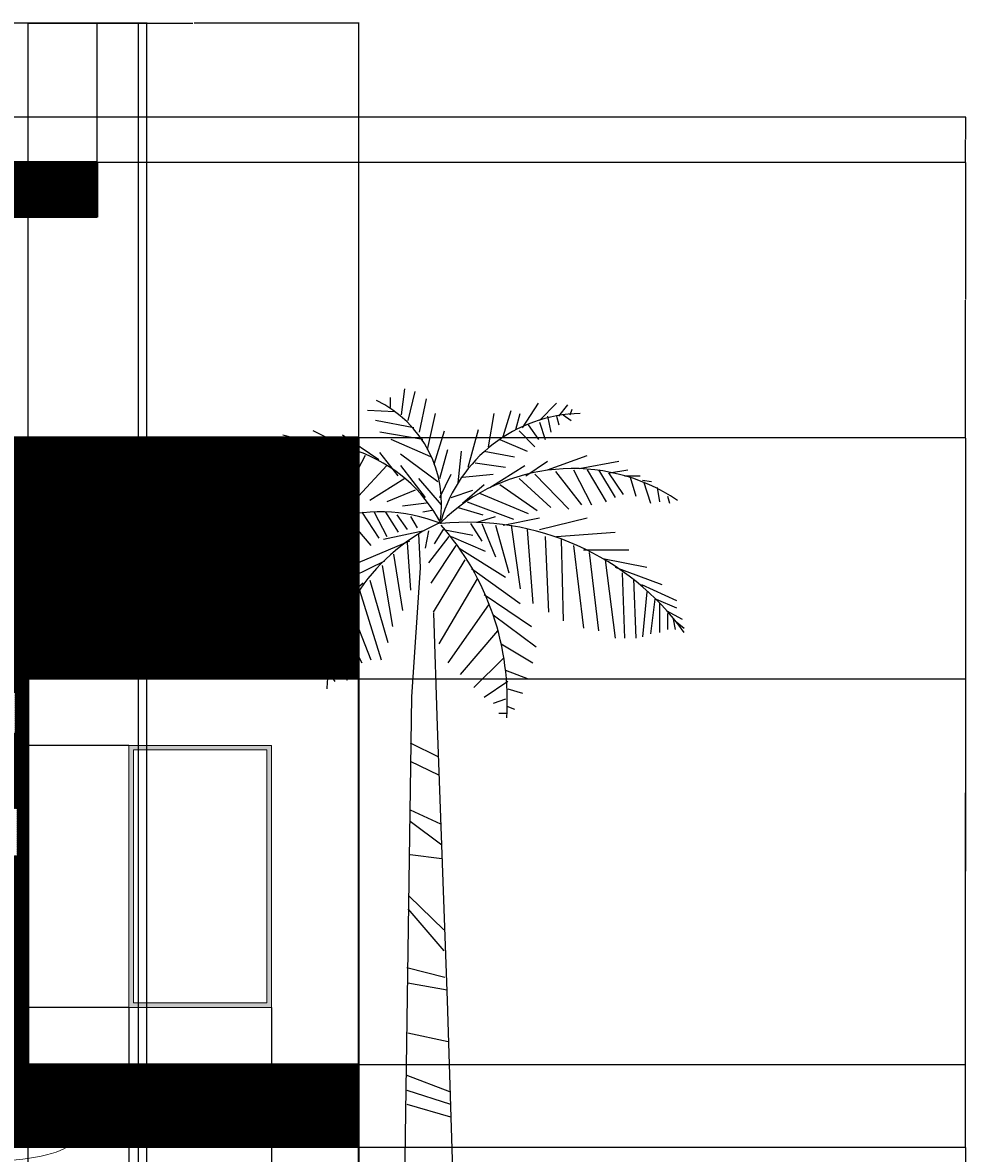
# Model space of a CAD drawing. Units: inches. Extents: x 484 to 1264, y 95 to 991.
# Tile 8 of 8: x 853 to 1264, y 499 to 991. Entities that reach past the tile are written whole.
import ezdxf

# ---------------------------------------------------------------- set-up
doc = ezdxf.new("R2010")
doc.units = ezdxf.units.IN
doc.header["$MEASUREMENT"] = 0
for name, color, linetype, lineweight in [('A-ANNO-DIMS', 2, 'Continuous', 18), ('A-ELEV-TRIM', 7, 'Continuous', 18), ('A-GLAZ', 7, 'Continuous', 18), ('A-WALL', 7, 'Continuous', 35)]:
    doc.layers.add(name, color=color, linetype=linetype, lineweight=lineweight)
doc.layers.add('A-ELEV-TRIM-PATT', color=40, linetype='Continuous', lineweight=13, true_color=0xe7c208)
doc.layers.add('A-WALL-FRAM-PATT', color=158, linetype='Continuous', lineweight=13, true_color=0x131d3e)
doc.layers.add('TREES', color=92, linetype='Continuous')
doc.styles.get("Standard").update_dxf_attribs({"font": 'arial.ttf'})
doc.dimstyles.get("Standard").update_dxf_attribs({"dimtxt": 0.18, "dimasz": 0.18, "dimexe": 0.18, "dimexo": 0.0625, "dimgap": 0.09, "dimtad": 0, "dimtih": 1, "dimtoh": 1, "dimdec": 4, "dimzin": 0, "dimdsep": 46, "dimtxsty": 'Standard', "dimcen": 0.09, "dimadec": 0, "dimazin": 0, "dimtfac": 1, "dimtdec": 4, "dimtofl": 0, "dimtmove": 0, "dimatfit": 3, "dimfxl": 1, "dimtolj": 1, "dimtzin": 0, "dimarcsym": 0})

# ---------------------------------------------------------------- blocks, each defined once
blk = doc.blocks.new('*U3')
for p, q in [((-5.567, 196.707), (-4.987, 201.167)), ((-7.5, 199.68), (-7.5, 197.946)), ((-4.407, 195.716), (-3.247, 200.672)), ((-2.474, 193.733), (-1.315, 199.433)), ((-6.727, 197.202), (-11.366, 197.45)), ((11.829, 192.99), (13.182, 197.45)), ((15.116, 194.477), (17.822, 198.689)), ((18.015, 195.716), (20.914, 198.689)), ((21.301, 196.459), (22.847, 198.441)), ((23.234, 196.707), (23.62, 197.698)), ((-3.441, 194.477), (-10.013, 195.716)), ((-1.121, 190.759), (0.232, 196.955)), ((9.317, 191.255), (10.283, 196.955)), ((13.956, 194.229), (14.729, 196.955)), ((18.015, 195.468), (18.981, 192.494)), ((19.368, 196.459), (19.948, 193.733)), ((20.914, 196.459), (21.301, 194.972)), ((22.074, 196.707), (23.427, 195.716)), ((-20.064, 191.751), (-25.863, 193.238)), ((-15.232, 191.255), (-20.644, 193.981)), ((-9.433, 189.025), (-15.618, 193.238)), ((-1.894, 192.494), (-9.24, 193.733)), ((0.038, 188.281), (1.778, 193.981)), ((5.837, 187.786), (7.577, 194.229)), ((14.536, 193.981), (17.242, 191.255)), ((16.082, 194.972), (17.822, 192.494)), ((-25.283, 191.751), (-29.342, 192.246)), ((-26.443, 191.503), (-26.636, 186.051)), ((-23.737, 191.751), (-24.51, 185.06)), ((-21.031, 191.998), (-21.804, 183.325)), ((-17.551, 191.503), (-20.451, 181.343)), ((-0.541, 189.52), (-7.307, 192.494)), ((11.25, 192.494), (15.889, 190.512)), ((-29.729, 190.759), (-31.469, 191.255)), ((-30.309, 190.512), (-30.695, 189.025)), ((-28.763, 190.759), (-28.763, 188.281)), ((-14.265, 190.759), (-18.131, 182.086)), ((-11.753, 189.768), (-15.425, 182.83)), ((-6.147, 186.299), (-9.24, 190.264)), ((-5.76, 190.016), (0.618, 185.308)), ((1.005, 185.803), (2.358, 190.759)), ((4.098, 185.06), (4.678, 190.512)), ((8.544, 190.512), (13.763, 189.52)), ((19.368, 187.29), (26.133, 189.768)), ((-8.08, 188.034), (-12.912, 182.83)), ((-5.76, 188.034), (-1.508, 182.582)), ((6.997, 188.529), (12.216, 187.786)), ((9.51, 184.317), (15.502, 188.034)), ((15.695, 186.299), (19.368, 188.777)), ((24.78, 187.538), (31.546, 188.777)), ((-4.987, 185.803), (-10.979, 182.086)), ((-2.668, 185.803), (1.198, 181.343)), ((1.005, 182.582), (2.938, 186.547)), ((4.871, 186.051), (10.09, 186.547)), ((14.536, 185.803), (19.948, 180.847)), ((17.242, 186.547), (23.041, 180.599)), ((20.721, 187.042), (25.167, 181.343)), ((23.814, 187.29), (26.907, 181.343)), ((26.133, 187.29), (29.419, 181.838)), ((28.066, 187.29), (30.966, 182.582)), ((29.806, 186.795), (32.319, 183.078)), ((29.999, 186.795), (33.092, 187.29)), ((32.512, 186.299), (35.218, 186.299)), ((33.479, 186.051), (34.445, 182.83)), ((35.605, 185.556), (37.151, 185.308)), ((-3.247, 183.821), (-8.08, 181.838)), ((2.938, 182.582), (6.61, 183.821)), ((4.871, 181.591), (8.544, 184.812)), ((11.25, 184.812), (17.628, 180.352)), ((35.798, 185.308), (36.958, 181.591)), ((38.118, 184.317), (38.504, 181.838)), ((5.644, 181.838), (13.569, 178.865)), ((7.77, 183.325), (16.082, 179.856)), ((39.857, 182.83), (40.244, 181.591)), ((-12.332, 180.104), (-9.433, 175.643)), ((-10.206, 180.104), (-8.08, 175.891)), ((-8.273, 180.104), (-6.147, 176.635)), ((-1.315, 181.591), (-5.374, 181.095)), ((-0.348, 180.352), (-1.894, 180.104)), ((4.098, 180.847), (8.35, 179.608)), ((-15.618, 179.36), (-20.644, 178.617)), ((-17.358, 178.617), (-13.299, 173.661)), ((-15.038, 179.36), (-10.786, 174.404)), ((-6.34, 179.608), (-4.6, 177.13)), ((-4.021, 179.36), (-2.861, 177.378)), ((6.224, 178.121), (8.157, 175.148)), ((7.384, 178.369), (10.476, 179.36)), ((8.157, 178.121), (10.476, 172.422)), ((10.476, 177.874), (12.796, 169.696)), ((11.829, 177.874), (18.015, 179.113)), ((13.182, 177.874), (14.729, 166.97)), ((18.015, 177.13), (26.133, 179.113)), ((-21.031, 177.626), (-24.897, 176.387)), ((-24.317, 175.891), (-18.711, 168.457)), ((-22.191, 176.635), (-16.391, 169.448)), ((-20.064, 177.626), (-15.812, 172.67)), ((-1.701, 176.882), (-8.66, 175.396)), ((-2.668, 176.387), (-2.376, 170.594)), ((-0.928, 176.882), (-1.508, 173.909)), ((2.551, 175.891), (-0.928, 171.431)), ((1.585, 177.13), (0.038, 174.652)), ((1.585, 177.13), (6.61, 176.139)), ((2.938, 175.891), (8.737, 173.413)), ((15.889, 177.13), (16.855, 164.492)), ((18.981, 175.891), (19.561, 163.005)), ((20.914, 175.891), (30.966, 176.635)), ((-25.09, 175.148), (-28.376, 174.404)), ((-25.476, 174.652), (-21.224, 167.466)), ((-4.214, 175.148), (-14.072, 170.935)), ((-4.6, 174.9), (-4.021, 166.722)), ((3.711, 174.404), (-0.541, 167.961)), ((21.688, 175.396), (22.074, 161.518)), ((23.814, 174.404), (25.554, 160.279)), ((-28.956, 172.174), (-32.435, 170.192)), ((-27.409, 173.413), (-30.695, 172.67)), ((-27.989, 172.422), (-26.056, 166.227)), ((-26.829, 173.661), (-23.544, 167.218)), ((-6.92, 172.917), (-5.374, 163.253)), ((4.291, 173.909), (12.216, 168.953)), ((25.554, 173.661), (33.285, 173.661)), ((26.52, 173.165), (28.066, 159.784)), ((28.839, 172.174), (36.378, 170.687)), ((-29.922, 170.687), (-27.989, 165.235)), ((-8.466, 171.678), (-16.585, 167.713)), ((-8.853, 170.935), (-7.113, 160.527)), ((5.257, 171.926), (-0.155, 163.005)), ((6.417, 170.439), (14.729, 164.492)), ((29.226, 171.926), (30.966, 158.545)), ((30.966, 170.687), (38.891, 167.713)), ((-31.082, 169.944), (-32.435, 169.2)), ((-31.662, 168.705), (-31.082, 165.483)), ((-10.979, 168.457), (-7.887, 157.801)), ((7.384, 168.705), (0.812, 157.553)), ((32.126, 169.696), (32.512, 158.545)), ((34.058, 168.705), (34.445, 158.545)), ((-32.628, 167.961), (-33.208, 167.961)), ((-32.628, 167.713), (-32.435, 165.979)), ((-12.139, 167.961), (-19.098, 162.014)), ((-12.719, 166.722), (-9.046, 154.828)), ((35.412, 167.713), (41.404, 164.988)), ((36.378, 166.474), (35.605, 158.792)), ((8.544, 165.979), (16.662, 160.527)), ((37.731, 165.235), (36.958, 159.288)), ((37.924, 165.235), (41.404, 163.749)), ((38.504, 164.492), (38.504, 159.536)), ((-14.265, 164.244), (-19.678, 158.049)), ((-14.265, 163.749), (-10.786, 154.828)), ((9.317, 164.244), (2.358, 154.332)), ((10.09, 162.51), (17.435, 157.058)), ((39.664, 163.253), (42.37, 161.766)), ((39.857, 162.757), (39.857, 160.031)), ((-15.618, 160.775), (-12.332, 154.332)), ((40.824, 161.766), (41.21, 160.031)), ((41.21, 161.518), (42.757, 160.279)), ((-16.005, 160.031), (-19.484, 154.084)), ((-16.585, 158.545), (-13.106, 152.35)), ((10.863, 159.784), (4.484, 152.35)), ((11.443, 157.553), (16.855, 154.332)), ((-17.358, 155.819), (-14.845, 151.358)), ((11.829, 155.075), (6.804, 150.119)), ((-18.131, 153.589), (-19.484, 151.606)), ((12.216, 153.093), (16.082, 151.606)), ((-17.938, 152.597), (-16.972, 151.111)), ((12.603, 151.111), (8.544, 148.385)), ((12.603, 149.872), (15.116, 149.128)), ((12.216, 148.137), (10.09, 147.393)), ((12.409, 146.898), (13.763, 146.402)), ((12.409, 145.659), (11.056, 145.659)), ((-4.081, 140.645), (0.753, 138.261)), ((-4.081, 137.547), (0.753, 135.163)), ((-4.081, 129.205), (1.124, 126.821)), ((-4.081, 127.298), (1.31, 123.246)), ((-4.081, 121.578), (1.31, 120.863)), ((-4.267, 114.428), (1.682, 108.708)), ((-4.453, 112.283), (1.682, 105.133)), ((-4.639, 102.273), (1.868, 100.604)), ((-4.453, 99.651), (2.24, 98.459)), ((-4.453, 91.071), (2.426, 89.641)), ((-4.825, 83.921), (2.612, 81.061)), ((-4.639, 81.299), (2.797, 78.916)), ((-4.639, 78.916), (2.797, 76.771))]:
    blk.add_line(p, q)
for points in [[(-2.363, 170.553), (-3.88, 148.505), (-4.988, 69.634), (-3.325, 24.869), (0, 0)], [(-0.116, 162.848), (0.554, 143.532), (2.217, 96.635), (3.88, 44.054), (7.76, 12.079), (11.64, 0)]]:
    blk.add_lwpolyline(points)
for centre, radius, start, end in [((-18.427, 181.448), 19.715, 350.285, 64.11229), ((25.595, 171.567), 25.395, 91.40319, 163.882), ((-21.738, 166.094), 25.899, 27.67115, 112.5305), ((23.687, 155.341), 32.188, 56.19272, 134.3213), ((-9.259, 151.732), 28.386, 68.38311, 147.5322), ((14.394, 148.393), 32.752, 113.7592, 177.4133), ((5.828, 132.718), 45.639, 35.98777, 95.82273), ((-32.8, 147.923), 45.309, 356.1943, 41.37848)]:
    blk.add_arc(centre, radius, start, end)
blk = doc.blocks.new('*D18')
at = {"layer": 'A-ANNO-DIMS', "color": 0, "lineweight": -2, "transparency": 16777216}
for p, q in [((999.88, 501.38), (1264.08, 501.38)), ((1263.9, 501.2), (1263.9, 404.07)), ((1263.9, 306.56), (1263.9, 403.7)), ((595.38, 306.38), (1264.08, 306.38))]:
    blk.add_line(p, q, dxfattribs=at)
at = {"layer": 'A-ANNO-DIMS', "color": 0, "transparency": 16777216}
for points in [[(1263.87, 501.2), (1263.93, 501.2), (1263.9, 501.38)], [(1263.87, 306.56), (1263.93, 306.56), (1263.9, 306.38)]]:
    blk.add_solid(points, dxfattribs=at)
at = {"layer": 'Defpoints', "color": 0, "transparency": 16777216}
for p in [(999.81, 501.38), (1263.9, 501.38), (595.32, 306.38)]:
    blk.add_point(p, dxfattribs=at)
at = {"layer": 'A-ANNO-DIMS', "color": 0, "transparency": 16777216, "insert": (1263.9, 403.88), "char_height": 0.18, "attachment_point": 5}
blk.add_mtext('\\A1;195', dxfattribs=at)
blk = doc.blocks.new('*D19')
at = {"layer": 'A-ANNO-DIMS', "color": 0, "lineweight": -2, "transparency": 16777216}
for p, q in [((999.88, 810.38), (1264.08, 810.38)), ((1263.9, 810.2), (1263.9, 656.07)), ((1263.9, 501.56), (1263.9, 655.7)), ((999.88, 501.38), (1264.08, 501.38))]:
    blk.add_line(p, q, dxfattribs=at)
at = {"layer": 'A-ANNO-DIMS', "color": 0, "transparency": 16777216}
for points in [[(1263.87, 810.2), (1263.93, 810.2), (1263.9, 810.38)], [(1263.87, 501.56), (1263.93, 501.56), (1263.9, 501.38)]]:
    blk.add_solid(points, dxfattribs=at)
at = {"layer": 'Defpoints', "color": 0, "transparency": 16777216}
for p in [(999.81, 810.38), (1263.9, 810.38), (999.81, 501.38)]:
    blk.add_point(p, dxfattribs=at)
at = {"layer": 'A-ANNO-DIMS', "color": 0, "transparency": 16777216, "insert": (1263.9, 655.88), "char_height": 0.18, "attachment_point": 5}
blk.add_mtext('\\A1;309', dxfattribs=at)
blk = doc.blocks.new('*D20')
at = {"layer": 'A-ANNO-DIMS', "color": 0, "lineweight": -2, "transparency": 16777216}
for p, q in [((885.88, 930.38), (1264.08, 930.38)), ((1263.9, 930.2), (1263.9, 870.57)), ((1263.9, 810.56), (1263.9, 870.2)), ((999.88, 810.38), (1264.08, 810.38))]:
    blk.add_line(p, q, dxfattribs=at)
at = {"layer": 'A-ANNO-DIMS', "color": 0, "transparency": 16777216}
for points in [[(1263.87, 930.2), (1263.93, 930.2), (1263.9, 930.38)], [(1263.87, 810.56), (1263.93, 810.56), (1263.9, 810.38)]]:
    blk.add_solid(points, dxfattribs=at)
at = {"layer": 'Defpoints', "color": 0, "transparency": 16777216}
for p in [(885.81, 930.38), (1263.9, 930.38), (999.81, 810.38)]:
    blk.add_point(p, dxfattribs=at)
at = {"layer": 'A-ANNO-DIMS', "color": 0, "transparency": 16777216, "insert": (1263.9, 870.38), "char_height": 0.18, "attachment_point": 5}
blk.add_mtext('\\A1;120', dxfattribs=at)
blk = doc.blocks.new('*D22')
at = {"layer": 'A-ANNO-DIMS', "color": 0, "lineweight": -2, "transparency": 16777216}
for p, q in [((639.81, 930.45), (639.81, 991.11)), ((639.99, 990.93), (762.52, 990.93)), ((885.63, 990.93), (763.11, 990.93)), ((885.81, 930.45), (885.81, 991.11))]:
    blk.add_line(p, q, dxfattribs=at)
at = {"layer": 'A-ANNO-DIMS', "color": 0, "transparency": 16777216}
for points in [[(639.99, 990.96), (639.99, 990.9), (639.81, 990.93)], [(885.63, 990.96), (885.63, 990.9), (885.81, 990.93)]]:
    blk.add_solid(points, dxfattribs=at)
at = {"layer": 'Defpoints', "color": 0, "transparency": 16777216}
for p in [(885.81, 990.93), (639.81, 930.38), (885.81, 930.38)]:
    blk.add_point(p, dxfattribs=at)
at = {"layer": 'A-ANNO-DIMS', "color": 0, "transparency": 16777216, "insert": (762.81, 990.93), "char_height": 0.18, "attachment_point": 5}
blk.add_mtext('\\A1;246', dxfattribs=at)
blk = doc.blocks.new('*D31')
at = {"layer": 'A-ANNO-DIMS', "color": 0, "lineweight": -2, "transparency": 16777216}
for p, q in [((760.93, 950.08), (1264.08, 950.08)), ((1263.9, 949.9), (1263.9, 940.41)), ((1263.9, 930.56), (1263.9, 940.05)), ((885.88, 930.38), (1264.08, 930.38))]:
    blk.add_line(p, q, dxfattribs=at)
at = {"layer": 'A-ANNO-DIMS', "color": 0, "transparency": 16777216}
for points in [[(1263.87, 949.9), (1263.93, 949.9), (1263.9, 950.08)], [(1263.87, 930.56), (1263.93, 930.56), (1263.9, 930.38)]]:
    blk.add_solid(points, dxfattribs=at)
at = {"layer": 'Defpoints', "color": 0, "transparency": 16777216}
for p in [(760.87, 950.08), (1263.9, 950.08), (885.81, 930.38)]:
    blk.add_point(p, dxfattribs=at)
at = {"layer": 'A-ANNO-DIMS', "color": 0, "transparency": 16777216, "insert": (1263.9, 940.23), "char_height": 0.18, "attachment_point": 5}
blk.add_mtext('\\A1;19.694', dxfattribs=at)
blk = doc.blocks.new('*D32')
at = {"layer": 'A-ANNO-DIMS', "color": 0, "lineweight": -2, "transparency": 16777216}
for p, q in [((885.75, 930.38), (484.15, 930.38)), ((484.33, 930.2), (484.33, 918.56)), ((484.33, 906.56), (484.33, 918.2)), ((885.75, 906.38), (484.15, 906.38))]:
    blk.add_line(p, q, dxfattribs=at)
at = {"layer": 'A-ANNO-DIMS', "color": 0, "transparency": 16777216}
for points in [[(484.3, 930.2), (484.36, 930.2), (484.33, 930.38)], [(484.3, 906.56), (484.36, 906.56), (484.33, 906.38)]]:
    blk.add_solid(points, dxfattribs=at)
at = {"layer": 'Defpoints', "color": 0, "transparency": 16777216}
for p in [(484.33, 930.38), (885.81, 930.38), (885.81, 906.38)]:
    blk.add_point(p, dxfattribs=at)
at = {"layer": 'A-ANNO-DIMS', "color": 0, "transparency": 16777216, "insert": (484.33, 918.38), "char_height": 0.18, "attachment_point": 5}
blk.add_mtext('\\A1;24', dxfattribs=at)
blk = doc.blocks.new('*D38')
at = {"layer": 'A-ANNO-DIMS', "color": 0, "lineweight": -2, "transparency": 16777216}
for p, q in [((899.62, 676.35), (484.15, 676.35)), ((484.33, 676.17), (484.33, 619.48)), ((484.33, 562.44), (484.33, 619.12)), ((899.62, 562.26), (484.15, 562.26))]:
    blk.add_line(p, q, dxfattribs=at)
at = {"layer": 'A-ANNO-DIMS', "color": 0, "transparency": 16777216}
for points in [[(484.3, 676.17), (484.36, 676.17), (484.33, 676.35)], [(484.3, 562.44), (484.36, 562.44), (484.33, 562.26)]]:
    blk.add_solid(points, dxfattribs=at)
at = {"layer": 'Defpoints', "color": 0, "transparency": 16777216}
for p in [(484.33, 676.35), (899.68, 676.35), (899.68, 562.26)]:
    blk.add_point(p, dxfattribs=at)
at = {"layer": 'A-ANNO-DIMS', "color": 0, "transparency": 16777216, "insert": (484.33, 619.3), "char_height": 0.18, "attachment_point": 5}
blk.add_mtext('\\A1;114.1', dxfattribs=at)
blk = doc.blocks.new('*D39')
at = {"layer": 'A-ANNO-DIMS', "color": 0, "lineweight": -2, "transparency": 16777216}
for p, q in [((899.62, 562.26), (484.15, 562.26)), ((484.33, 562.08), (484.33, 550)), ((484.33, 537.56), (484.33, 549.64)), ((855.75, 537.38), (484.15, 537.38))]:
    blk.add_line(p, q, dxfattribs=at)
at = {"layer": 'A-ANNO-DIMS', "color": 0, "transparency": 16777216}
for points in [[(484.3, 562.08), (484.36, 562.08), (484.33, 562.26)], [(484.3, 537.56), (484.36, 537.56), (484.33, 537.38)]]:
    blk.add_solid(points, dxfattribs=at)
at = {"layer": 'Defpoints', "color": 0, "transparency": 16777216}
for p in [(484.33, 562.26), (899.68, 562.26), (855.81, 537.38)]:
    blk.add_point(p, dxfattribs=at)
at = {"layer": 'A-ANNO-DIMS', "color": 0, "transparency": 16777216, "insert": (484.33, 549.82), "char_height": 0.18, "attachment_point": 5}
blk.add_mtext('\\A1;24.87', dxfattribs=at)
blk = doc.blocks.new('*D40')
at = {"layer": 'A-ANNO-DIMS', "color": 0, "lineweight": -2, "transparency": 16777216}
for p, q in [((899.68, 562.19), (899.68, 94.79)), ((961.76, 562.19), (961.76, 94.79)), ((899.86, 94.97), (930.33, 94.97)), ((961.58, 94.97), (931.12, 94.97))]:
    blk.add_line(p, q, dxfattribs=at)
at = {"layer": 'A-ANNO-DIMS', "color": 0, "transparency": 16777216}
for points in [[(899.86, 95), (899.86, 94.94), (899.68, 94.97)], [(961.58, 95), (961.58, 94.94), (961.76, 94.97)]]:
    blk.add_solid(points, dxfattribs=at)
at = {"layer": 'Defpoints', "color": 0, "transparency": 16777216}
for p in [(899.68, 562.26), (961.76, 562.26), (961.76, 94.97)]:
    blk.add_point(p, dxfattribs=at)
at = {"layer": 'A-ANNO-DIMS', "color": 0, "transparency": 16777216, "insert": (930.72, 94.97), "char_height": 0.18, "attachment_point": 5}
blk.add_mtext('\\A1;62.08', dxfattribs=at)
blk = doc.blocks.new('*D41')
at = {"layer": 'A-ANNO-DIMS', "color": 0, "lineweight": -2, "transparency": 16777216}
for p, q in [((961.76, 562.19), (961.76, 94.79)), ((999.81, 537.32), (999.81, 94.79)), ((961.94, 94.97), (980.39, 94.97)), ((999.63, 94.97), (981.18, 94.97))]:
    blk.add_line(p, q, dxfattribs=at)
at = {"layer": 'A-ANNO-DIMS', "color": 0, "transparency": 16777216}
for points in [[(961.94, 95), (961.94, 94.94), (961.76, 94.97)], [(999.63, 95), (999.63, 94.94), (999.81, 94.97)]]:
    blk.add_solid(points, dxfattribs=at)
at = {"layer": 'Defpoints', "color": 0, "transparency": 16777216}
for p in [(961.76, 562.26), (999.81, 537.38), (999.81, 94.97)]:
    blk.add_point(p, dxfattribs=at)
at = {"layer": 'A-ANNO-DIMS', "color": 0, "transparency": 16777216, "insert": (980.79, 94.97), "char_height": 0.18, "attachment_point": 5}
blk.add_mtext('\\A1;38.05', dxfattribs=at)
blk = doc.blocks.new('*D42')
at = {"layer": 'A-ANNO-DIMS', "color": 0, "lineweight": -2, "transparency": 16777216}
for p, q in [((855.81, 705.45), (855.81, 991.11)), ((855.99, 990.93), (927.53, 990.93)), ((999.63, 990.93), (928.09, 990.93)), ((999.81, 705.45), (999.81, 991.11))]:
    blk.add_line(p, q, dxfattribs=at)
at = {"layer": 'A-ANNO-DIMS', "color": 0, "transparency": 16777216}
for points in [[(855.99, 990.96), (855.99, 990.9), (855.81, 990.93)], [(999.63, 990.96), (999.63, 990.9), (999.81, 990.93)]]:
    blk.add_solid(points, dxfattribs=at)
at = {"layer": 'Defpoints', "color": 0, "transparency": 16777216}
for p in [(999.81, 990.93), (855.81, 705.38), (999.81, 705.38)]:
    blk.add_point(p, dxfattribs=at)
at = {"layer": 'A-ANNO-DIMS', "color": 0, "transparency": 16777216, "insert": (927.81, 990.93), "char_height": 0.18, "attachment_point": 5}
blk.add_mtext('\\A1;144', dxfattribs=at)
blk = doc.blocks.new('*D43')
at = {"layer": 'A-ANNO-DIMS', "color": 0, "lineweight": -2, "transparency": 16777216}
for p, q in [((855.88, 705.38), (1264.08, 705.38)), ((1263.9, 705.2), (1263.9, 621.57)), ((1263.9, 537.56), (1263.9, 621.2)), ((855.88, 537.38), (1264.08, 537.38))]:
    blk.add_line(p, q, dxfattribs=at)
at = {"layer": 'A-ANNO-DIMS', "color": 0, "transparency": 16777216}
for points in [[(1263.87, 705.2), (1263.93, 705.2), (1263.9, 705.38)], [(1263.87, 537.56), (1263.93, 537.56), (1263.9, 537.38)]]:
    blk.add_solid(points, dxfattribs=at)
at = {"layer": 'Defpoints', "color": 0, "transparency": 16777216}
for p in [(855.81, 705.38), (1263.9, 705.38), (855.81, 537.38)]:
    blk.add_point(p, dxfattribs=at)
at = {"layer": 'A-ANNO-DIMS', "color": 0, "transparency": 16777216, "insert": (1263.9, 621.38), "char_height": 0.18, "attachment_point": 5}
blk.add_mtext('\\A1;168', dxfattribs=at)
blk = doc.blocks.new('*D44')
at = {"layer": 'A-ANNO-DIMS', "color": 0, "lineweight": -2, "transparency": 16777216}
for p, q in [((999.75, 537.38), (484.15, 537.38)), ((484.33, 537.2), (484.33, 519.57)), ((484.33, 501.56), (484.33, 519.2)), ((999.75, 501.38), (484.15, 501.38))]:
    blk.add_line(p, q, dxfattribs=at)
at = {"layer": 'A-ANNO-DIMS', "color": 0, "transparency": 16777216}
for points in [[(484.3, 537.2), (484.36, 537.2), (484.33, 537.38)], [(484.3, 501.56), (484.36, 501.56), (484.33, 501.38)]]:
    blk.add_solid(points, dxfattribs=at)
at = {"layer": 'Defpoints', "color": 0, "transparency": 16777216}
for p in [(484.33, 537.38), (999.81, 537.38), (999.81, 501.38)]:
    blk.add_point(p, dxfattribs=at)
at = {"layer": 'A-ANNO-DIMS', "color": 0, "transparency": 16777216, "insert": (484.33, 519.38), "char_height": 0.18, "attachment_point": 5}
blk.add_mtext('\\A1;36', dxfattribs=at)
blk = doc.blocks.new('*D54')
at = {"layer": 'A-ANNO-DIMS', "color": 0, "lineweight": -2, "transparency": 16777216}
for p, q in [((831.81, 420.5), (831.81, 991.11)), ((831.99, 990.93), (843.59, 990.93)), ((855.63, 990.93), (844.03, 990.93)), ((855.81, 420.5), (855.81, 991.11))]:
    blk.add_line(p, q, dxfattribs=at)
at = {"layer": 'A-ANNO-DIMS', "color": 0, "transparency": 16777216}
for points in [[(831.99, 990.96), (831.99, 990.9), (831.81, 990.93)], [(855.63, 990.96), (855.63, 990.9), (855.81, 990.93)]]:
    blk.add_solid(points, dxfattribs=at)
at = {"layer": 'Defpoints', "color": 0, "transparency": 16777216}
for p in [(855.81, 990.93), (831.81, 420.44), (855.81, 420.44)]:
    blk.add_point(p, dxfattribs=at)
at = {"layer": 'A-ANNO-DIMS', "color": 0, "transparency": 16777216, "insert": (843.81, 990.93), "char_height": 0.18, "attachment_point": 5}
blk.add_mtext('\\A1;24', dxfattribs=at)
blk = doc.blocks.new('*D57')
at = {"layer": 'A-ANNO-DIMS', "color": 0, "lineweight": -2, "transparency": 16777216}
for p, q in [((855.81, 396.45), (855.81, 991.11)), ((855.99, 990.93), (879.59, 990.93)), ((903.63, 990.93), (880.04, 990.93)), ((903.81, 396.45), (903.81, 991.11))]:
    blk.add_line(p, q, dxfattribs=at)
at = {"layer": 'A-ANNO-DIMS', "color": 0, "transparency": 16777216}
for points in [[(855.99, 990.96), (855.99, 990.9), (855.81, 990.93)], [(903.63, 990.96), (903.63, 990.9), (903.81, 990.93)]]:
    blk.add_solid(points, dxfattribs=at)
at = {"layer": 'Defpoints', "color": 0, "transparency": 16777216}
for p in [(903.81, 990.93), (855.81, 396.38), (903.81, 396.38)]:
    blk.add_point(p, dxfattribs=at)
at = {"layer": 'A-ANNO-DIMS', "color": 0, "transparency": 16777216, "insert": (879.81, 990.93), "char_height": 0.18, "attachment_point": 5}
blk.add_mtext('\\A1;48', dxfattribs=at)
blk = doc.blocks.new('*D61')
at = {"layer": 'A-ANNO-DIMS', "color": 0, "lineweight": -2, "transparency": 16777216}
for p, q in [((855.81, 396.45), (855.81, 991.11)), ((855.99, 990.93), (881.26, 990.93)), ((907.32, 990.93), (882.05, 990.93)), ((907.5, 442.84), (907.5, 991.11))]:
    blk.add_line(p, q, dxfattribs=at)
at = {"layer": 'A-ANNO-DIMS', "color": 0, "transparency": 16777216}
for points in [[(855.99, 990.96), (855.99, 990.9), (855.81, 990.93)], [(907.32, 990.96), (907.32, 990.9), (907.5, 990.93)]]:
    blk.add_solid(points, dxfattribs=at)
at = {"layer": 'Defpoints', "color": 0, "transparency": 16777216}
for p in [(907.5, 990.93), (907.5, 442.78), (855.81, 396.38)]:
    blk.add_point(p, dxfattribs=at)
at = {"layer": 'A-ANNO-DIMS', "color": 0, "transparency": 16777216, "insert": (881.66, 990.93), "char_height": 0.18, "attachment_point": 5}
blk.add_mtext('\\A1;51.68', dxfattribs=at)

msp = doc.modelspace()

# ---------------------------------------------------------------- hatches: boundary and pattern name
at = {"layer": 'A-ELEV-TRIM-PATT'}
h = msp.add_hatch(color=256, dxfattribs=at)
h.dxf.hatch_style = 1
h.paths.add_polyline_path([(961.7639, 676.3493), (899.6817, 676.3493), (899.6817, 562.256), (961.7639, 562.256)])
h.paths.add_polyline_path([(901.6817, 674.3493), (959.7639, 674.3493), (959.7639, 564.256), (901.6817, 564.256)], flags=16)
at = {"layer": 'A-WALL-FRAM-PATT'}
h = msp.add_hatch(dxfattribs=at)
h.set_pattern_fill('ANSI31', color=256)
h.paths.add_polyline_path([(999.8147, 810.3846), (831.8147, 810.3846), (831.8147, 501.3846), (999.8147, 501.3846), (999.8147, 537.3846), (855.8147, 537.3846), (855.8147, 705.3846), (999.8147, 705.3846)])
h.paths.add_polyline_path([(850.1752, 699.3334), (850.1752, 681.6082), (840.6401, 681.6082), (840.6401, 699.3334)], flags=16)
h.paths.add_polyline_path([(850.9809, 648.8447), (850.9809, 628.2143), (839.9453, 628.2143), (839.9453, 648.8447)], flags=16)
h.paths.add_polyline_path([(849.208, 595.8059), (849.208, 577.6654), (838.5284, 577.6654), (838.5284, 595.8059)], flags=16)
h.paths.add_polyline_path([(663.8147, 906.3846), (709.0683, 906.3846), (709.0683, 930.3846), (639.8147, 930.3846), (639.8147, 408.3846), (663.8147, 408.3846)])
h.paths.add_polyline_path([(885.8147, 930.3846), (775.2587, 930.3846), (775.2587, 906.3846), (885.8147, 906.3846)])
h.paths.add_polyline_path([(760.8695, 930.3846), (750.5092, 930.3846), (750.5092, 906.3846), (760.8695, 906.3846)])
h.paths.add_polyline_path([(736.12, 930.3846), (723.4575, 930.3846), (723.4575, 906.3846), (736.12, 906.3846)])

# ---------------------------------------------------------------- linework, layer by layer
at = {"layer": 'A-ELEV-TRIM'}
msp.add_ellipse((839.1596, 504.6689), major_axis=(-35.8241, 0), ratio=0.25748145, start_param=1.36430507, end_param=2.77754981, dxfattribs=at)
at = {"layer": 'A-GLAZ'}
for points in [[(899.6817, 676.3493), (961.7639, 676.3493), (961.7639, 562.256), (899.6817, 562.256)], [(901.6817, 674.3493), (959.7639, 674.3493), (959.7639, 564.256), (901.6817, 564.256)]]:
    msp.add_lwpolyline(points, close=True, dxfattribs=at)
at = {"layer": 'A-WALL'}
for p, q in [((885.8147, 930.3846), (775.2587, 930.3846)), ((885.8147, 930.3846), (885.8147, 906.3846)), ((885.8147, 906.3846), (775.2587, 906.3846)), ((999.8147, 810.3846), (663.8147, 810.3846)), ((999.8147, 426.86), (999.8147, 810.3846)), ((999.8147, 705.3846), (855.8147, 705.3846)), ((855.8147, 705.3846), (855.8147, 537.3846)), ((999.8147, 537.3846), (855.8147, 537.3846)), ((999.8147, 501.3846), (663.8147, 501.3846))]:
    msp.add_line(p, q, dxfattribs=at)

# ---------------------------------------------------------------- block references
at = {"layer": 'TREES', "xscale": 2.548367839539612, "yscale": 2.548367839539612, "zscale": 2.548367839539612}
msp.add_blockref('*U3', (1032.522, 319.0159), dxfattribs=at)

# ---------------------------------------------------------------- dimensions: what is measured, and where the dimension line sits
at = {"layer": 'A-ANNO-DIMS'}
for base, p1, p2, override, picture, middle in [((885.8147, 990.929), (639.8147, 930.3846), (885.8147, 930.3846), {"dimdec": 0, "dimlfac": 1, "dimrnd": 0, "dimzin": 0, "dimdsep": 46, "dimlunit": 2}, '*D22', (762.8147, 990.929)), ((855.8147, 990.929), (831.8147, 420.4387), (855.8147, 420.4387), {"dimdec": 0, "dimlfac": 1, "dimrnd": 0, "dimzin": 0, "dimdsep": 46, "dimlunit": 2}, '*D54', (843.8147, 990.929)), ((999.8147, 990.929), (855.8147, 705.3846), (999.8147, 705.3846), {"dimdec": 0, "dimlfac": 1, "dimrnd": 0, "dimzin": 0, "dimdsep": 46, "dimlunit": 2}, '*D42', (927.8147, 990.929)), ((903.8147, 990.929), (855.8147, 396.3846), (903.8147, 396.3846), {"dimdec": 0, "dimlfac": 1, "dimrnd": 0, "dimzin": 0, "dimdsep": 46, "dimlunit": 2}, '*D57', (879.8147, 990.929)), ((907.4984, 990.929), (855.8147, 396.3846), (907.4984, 442.7783), {"dimdec": 2, "dimlfac": 1, "dimrnd": 0, "dimzin": 0, "dimdsep": 46, "dimlunit": 2}, '*D61', (881.6566, 990.929)), ((961.7639, 94.9714), (899.6817, 562.256), (961.7639, 562.256), {"dimdec": 2, "dimlfac": 1, "dimrnd": 0, "dimzin": 0, "dimdsep": 46, "dimlunit": 2}, '*D40', (930.7228, 94.9714)), ((999.8147, 94.9714), (961.7639, 562.256), (999.8147, 537.3846), {"dimdec": 2, "dimlfac": 1, "dimrnd": 0, "dimzin": 0, "dimdsep": 46, "dimlunit": 2}, '*D41', (980.7893, 94.9714))]:
    dim = msp.add_linear_dim(base=base, p1=p1, p2=p2, dimstyle='Standard', override=override, dxfattribs=at)
    dim.commit()
    dim.dimension.update_dxf_attribs({"geometry": picture, "text_midpoint": middle})
for base, p1, p2, override, picture, middle in [((1263.9032, 950.079), (885.8147, 930.3846), (760.8695, 950.079), {"dimdec": 3, "dimlfac": 1, "dimrnd": 0, "dimzin": 0, "dimdsep": 46, "dimlunit": 2}, '*D31', (1263.9032, 940.2318)), ((484.3261, 930.3846), (885.8147, 906.3846), (885.8147, 930.3846), {"dimdec": 0, "dimlfac": 1, "dimrnd": 0, "dimzin": 0, "dimdsep": 46, "dimlunit": 2}, '*D32', (484.3261, 918.3846)), ((1263.9032, 930.3846), (999.8147, 810.3846), (885.8147, 930.3846), {"dimdec": 0, "dimlfac": 1, "dimrnd": 0, "dimzin": 0, "dimdsep": 46, "dimlunit": 2}, '*D20', (1263.9032, 870.3846)), ((1263.9032, 810.3846), (999.8147, 501.3846), (999.8147, 810.3846), {"dimdec": 0, "dimlfac": 1, "dimrnd": 0, "dimzin": 0, "dimdsep": 46, "dimlunit": 2}, '*D19', (1263.9032, 655.8846)), ((1263.9032, 705.3846), (855.8147, 537.3846), (855.8147, 705.3846), {"dimdec": 0, "dimlfac": 1, "dimrnd": 0, "dimzin": 0, "dimdsep": 46, "dimlunit": 2}, '*D43', (1263.9032, 621.3846)), ((484.3261, 676.3493), (899.6817, 562.256), (899.6817, 676.3493), {"dimdec": 1, "dimlfac": 1, "dimrnd": 0, "dimzin": 0, "dimdsep": 46, "dimlunit": 2}, '*D38', (484.3261, 619.3026)), ((484.3261, 562.256), (855.8147, 537.3846), (899.6817, 562.256), {"dimdec": 2, "dimlfac": 1, "dimrnd": 0, "dimzin": 0, "dimdsep": 46, "dimlunit": 2}, '*D39', (484.3261, 549.8203)), ((484.3261, 537.3846), (999.8147, 501.3846), (999.8147, 537.3846), {"dimdec": 0, "dimlfac": 1, "dimrnd": 0, "dimzin": 0, "dimdsep": 46, "dimlunit": 2}, '*D44', (484.3261, 519.3846)), ((1263.9032, 501.3846), (595.3221, 306.3846), (999.8147, 501.3846), {"dimdec": 0, "dimlfac": 1, "dimrnd": 0, "dimzin": 0, "dimdsep": 46, "dimlunit": 2}, '*D18', (1263.9032, 403.8846))]:
    dim = msp.add_linear_dim(base=base, p1=p1, p2=p2, angle=90, dimstyle='Standard', override=override, dxfattribs=at)
    dim.commit()
    dim.dimension.update_dxf_attribs({"geometry": picture, "text_midpoint": middle})

doc.saveas('drawing.dxf')
